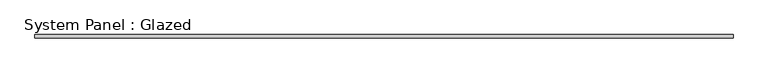
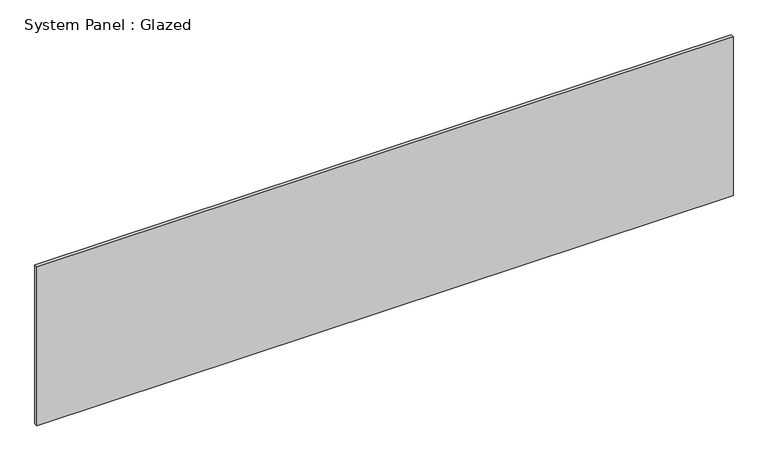
"""IFC4 building model written with IfcOpenShell, lengths in millimetres: plate geometry, System Panel : Glazed."""

from ifc_helpers import new_model, si_unit, origin, origin_with_axes, place, context, project, spatial, polyline, outline, extrude, source, transform, mapped, element, save


def system_panel_glazed_18441643(model_context):
    return source(origin(), model_context, "Body", "SweptSolid", [
        extrude(outline(polyline([(2528.6101998, 19.05), (-2528.6101998, 19.05), (-2528.6101998, 44.45), (2528.6101998, 44.45), (2528.6101998, 19.05)])), origin_with_axes(), (0.0, 0.0, 1.0), 1219.2),
    ])


if __name__ == "__main__":
    model = new_model("IFC4")
    model_context = context("Model", 3, world=origin())
    ifc_project = project(units=[si_unit("LENGTHUNIT", "METRE", prefix="MILLI")], contexts=[model_context])
    site = spatial("IfcSite", under=ifc_project)
    building = spatial("IfcBuilding", under=site)
    placement = place(None, origin())
    system_panel_glazed_shape = system_panel_glazed_18441643(model_context)
    element("IfcPlate", 1, ObjectType="System Panel : Glazed", at=placement, inside=building, context=model_context, shape_type="MappedRepresentation", body=[
        mapped(system_panel_glazed_shape, transform((0.0, 0.0, 0.0), x_axis=(1.0, 0.0, 0.0), y_axis=(0.0, 1.0, 0.0), z_axis=(0.0, 0.0, 1.0))),
    ])
    save(model, "model.ifc")

# Revit data of these elements
# Type "System Panel : Glazed"
#   Construction Type Id = "GSP4R"
#   Analytic Construction = "1/8 in Pilkington single glazing"
#   Visual Light Transmittance = 0.9
#   Solar Heat Gain Coefficient = 0.86
#   Heat Transfer Coefficient (U) = 1.18115 BTU/(h·ft²·°F)
# Element 1 (IfcPlate, "System Panel : Glazed")
#   Materials on its faces: "Glass"
# Materials
#   "Glass": class "Glass", colour RGB 0 128 192, transparency 0.75, Description = "Soda Lime Glass", Cost = 0
